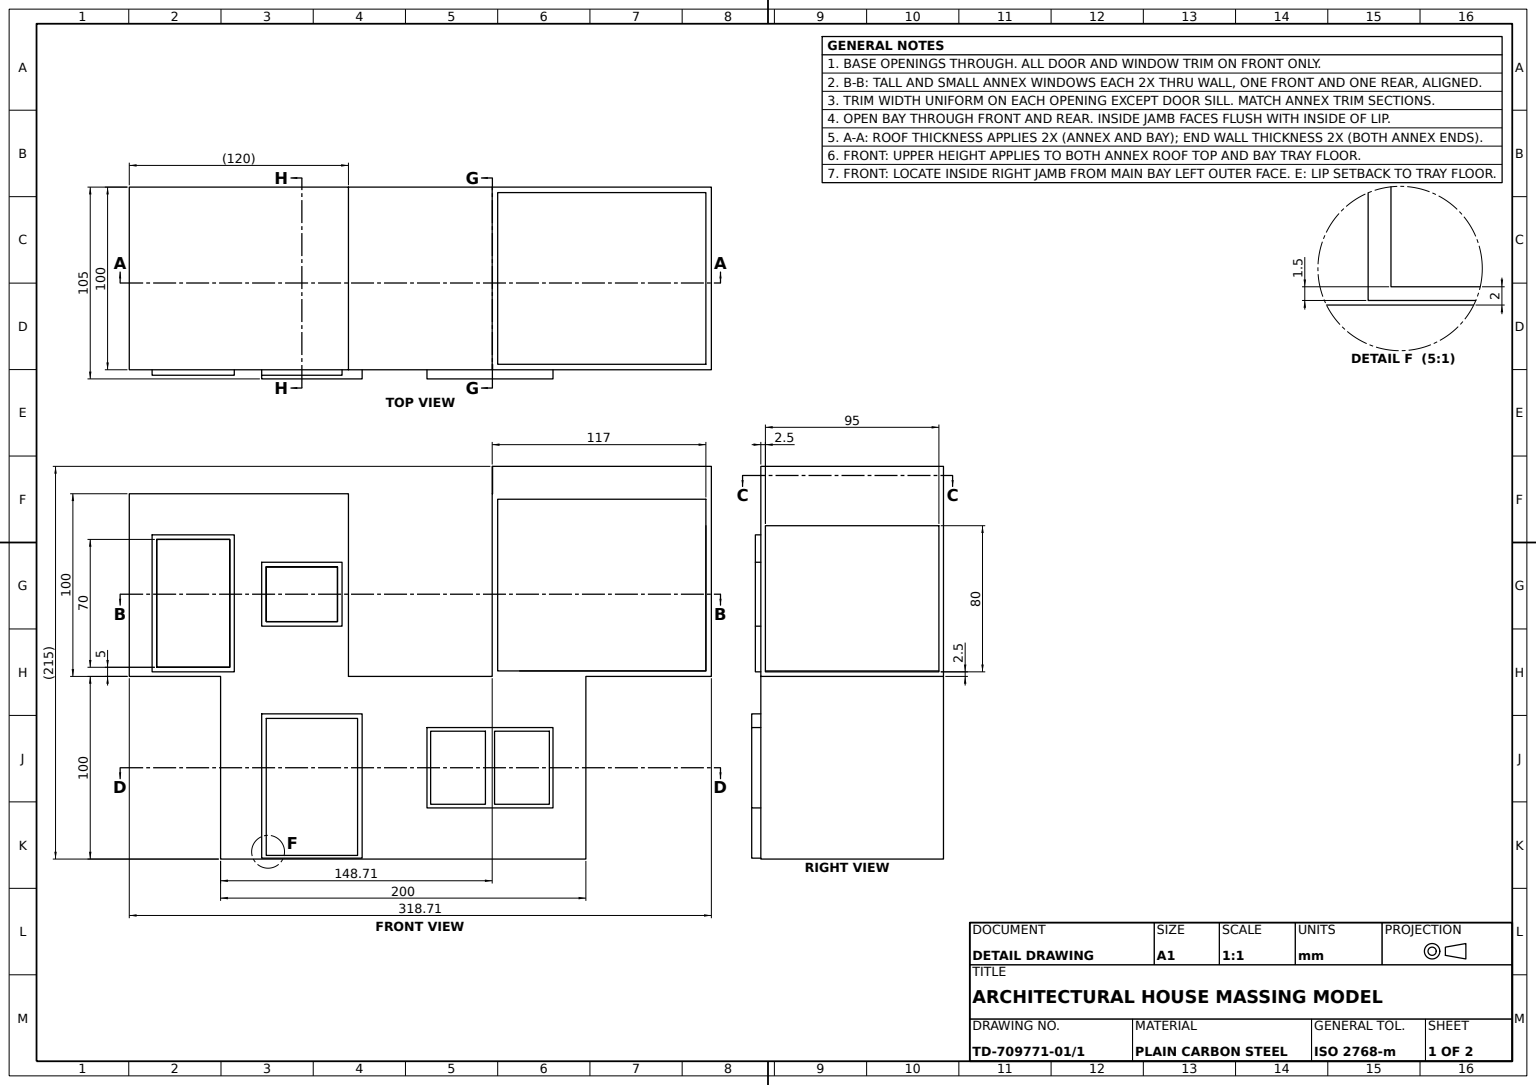
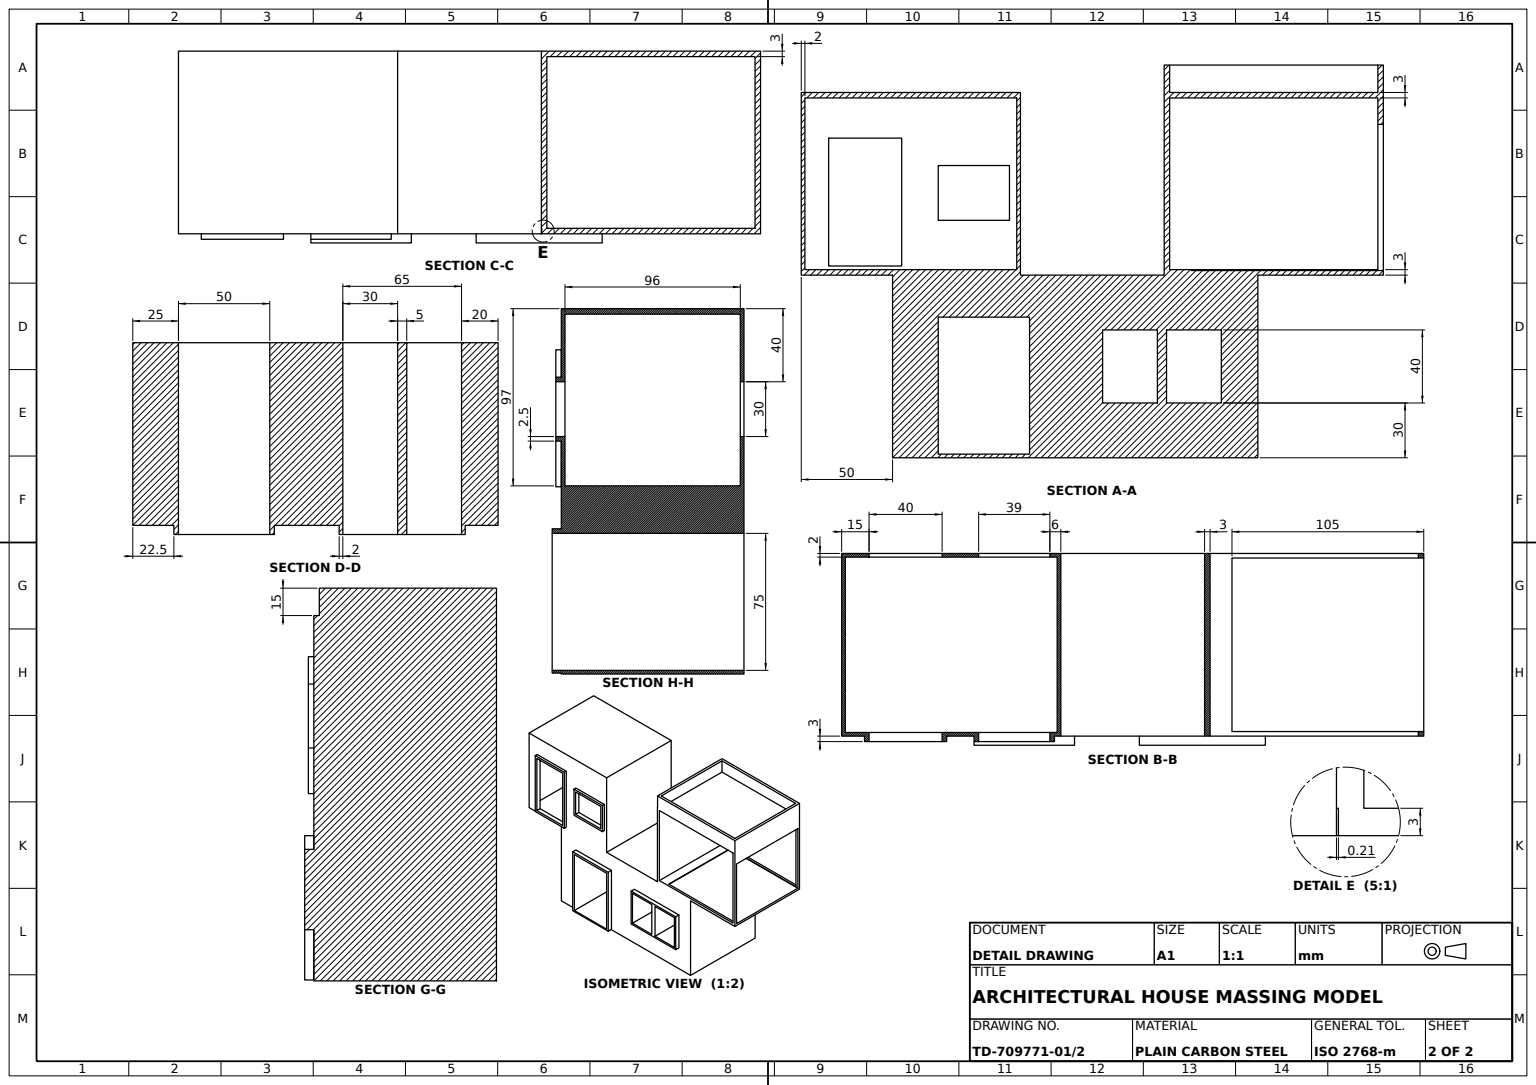
from build123d import *

# Parameters (mm, degrees)
BASE_BLOCK_SKETCH_W           = 200
BASE_BLOCK_SKETCH_H           = 100
BASE_BLOCK_DEPTH              = 100
UPPER_BLOCK_SKETCH_W          = 120
UPPER_BLOCK_SKETCH_H          = 100
UPPER_BLOCK_DEPTH             = 100
SIDE_ANNEX_DEPTH              = 100
FRONT_DOOR_OPENING_SKETCH_W   = 50
FRONT_DOOR_OPENING_SKETCH_H   = 75
FRONT_DOOR_OPENING_DEPTH      = 100
FRONT_WINDOW_OPENING_SKETCH_W = 65
FRONT_WINDOW_OPENING_SKETCH_H = 40
FRONT_WINDOW_OPENING_DEPTH    = 100
FRONT_WINDOW_MULLION_SKETCH_W = 5
FRONT_WINDOW_MULLION_SKETCH_H = 40
FRONT_WINDOW_MULLION_DEPTH    = 100
FRONT_WINDOW_FRAME_SKETCH_W   = 69
FRONT_WINDOW_FRAME_SKETCH_H   = 44
FRONT_WINDOW_FRAME_SKETCH_W_2 = 30
FRONT_WINDOW_FRAME_SKETCH_H_2 = 40
FRONT_WINDOW_FRAME_DEPTH      = 5
FRONT_DOOR_FRAME_SKETCH_W     = 55
FRONT_DOOR_FRAME_SKETCH_H     = 79
FRONT_DOOR_FRAME_SKETCH_W_2   = 50
FRONT_DOOR_FRAME_SKETCH_H_2   = 75
FRONT_DOOR_FRAME_DEPTH        = 5
UPPER_BLOCK_HOLLOW_SKETCH_W   = 114
UPPER_BLOCK_HOLLOW_SKETCH_H   = 94
UPPER_BLOCK_HOLLOW_DEPTH      = 125
UPPER_INTERIOR_CUT_SKETCH_W   = 95
UPPER_INTERIOR_CUT_SKETCH_H   = 80
UPPER_INTERIOR_CUT_DEPTH      = 105
UPPER_FRAME_MEMBER_1_SKETCH_W = 100
UPPER_FRAME_MEMBER_1_SKETCH_H = 15
UPPER_FRAME_MEMBER_1_DEPTH    = 3
UPPER_FRAME_MEMBER_2_SKETCH_W = 116.787548914
UPPER_FRAME_MEMBER_2_SKETCH_H = 15
UPPER_FRAME_MEMBER_2_DEPTH    = 3
UPPER_FRAME_MEMBER_3_SKETCH_W = 97
UPPER_FRAME_MEMBER_3_SKETCH_H = 15
UPPER_FRAME_MEMBER_3_DEPTH    = 3
UPPER_FRAME_MEMBER_4_SKETCH_W = 114
UPPER_FRAME_MEMBER_4_SKETCH_H = 15
UPPER_FRAME_MEMBER_4_DEPTH    = 3
ANNEX_DOOR_OPENING_SKETCH_W   = 40
ANNEX_DOOR_OPENING_SKETCH_H   = 70
ANNEX_DOOR_OPENING_DEPTH      = 153
ANNEX_WINDOW_OPENING_SKETCH_W = 39
ANNEX_WINDOW_OPENING_SKETCH_H = 30
ANNEX_WINDOW_OPENING_DEPTH    = 153
ANNEX_DOOR_FRAME_SKETCH_W     = 45
ANNEX_DOOR_FRAME_SKETCH_H     = 75
ANNEX_DOOR_FRAME_SKETCH_W_2   = 40
ANNEX_DOOR_FRAME_SKETCH_H_2   = 70
ANNEX_DOOR_FRAME_DEPTH        = 3
ANNEX_WINDOW_FRAME_SKETCH_W   = 44
ANNEX_WINDOW_FRAME_SKETCH_H   = 35
ANNEX_WINDOW_FRAME_SKETCH_W_2 = 39
ANNEX_WINDOW_FRAME_SKETCH_H_2 = 30
ANNEX_WINDOW_FRAME_DEPTH      = 3
ANNEX_HOLLOW_SKETCH_W         = 116
ANNEX_HOLLOW_SKETCH_H         = 96
ANNEX_HOLLOW_DEPTH            = 97
ANNEX_RIM_SKETCH_W            = 120
ANNEX_RIM_SKETCH_H            = 100
ANNEX_RIM_DEPTH               = 3


with BuildPart() as part:
    # Base Block Sketch → Base Block (new body)
    with BuildSketch(Plane(origin=(0, 0, 0), x_dir=(1, 0, 0), z_dir=(0, 1, 0))):
        with Locations((100, 50)):
            Rectangle(BASE_BLOCK_SKETCH_W, BASE_BLOCK_SKETCH_H)
    extrude(amount=BASE_BLOCK_DEPTH)

    # Upper Block Sketch → Upper Block (add)
    with BuildSketch(Plane(origin=(0, 100, 0), x_dir=(1, 0, 0), z_dir=(0, 1, 0))):
        with Locations((208.708454776, 50)):
            Rectangle(UPPER_BLOCK_SKETCH_W, UPPER_BLOCK_SKETCH_H)
    extrude(amount=UPPER_BLOCK_DEPTH)

    # Side Annex Sketch → Side Annex (add)
    with BuildSketch(Plane(origin=(0, 100, 0), x_dir=(1, 0, 0), z_dir=(0, 1, 0))):
        Polygon((0, 0), (70, 0), (70, 100), (0, 100), (-50, 100), (-50, 0), align=None)
    extrude(amount=SIDE_ANNEX_DEPTH)

    # Front Door Opening Sketch → Front Door Opening (cut)
    with BuildSketch(Plane.XY):
        with Locations((50, 39.5)):
            Rectangle(FRONT_DOOR_OPENING_SKETCH_W, FRONT_DOOR_OPENING_SKETCH_H)
    extrude(amount=-FRONT_DOOR_OPENING_DEPTH, mode=Mode.SUBTRACT)

    # Front Window Opening Sketch → Front Window Opening (cut)
    with BuildSketch(Plane.XY):
        with Locations((147.5, 50)):
            Rectangle(FRONT_WINDOW_OPENING_SKETCH_W, FRONT_WINDOW_OPENING_SKETCH_H)
    extrude(amount=-FRONT_WINDOW_OPENING_DEPTH, mode=Mode.SUBTRACT)

    # Front Window Mullion Sketch → Front Window Mullion (add)
    with BuildSketch(Plane.XY):
        with Locations((147.5, 50)):
            Rectangle(FRONT_WINDOW_MULLION_SKETCH_W, FRONT_WINDOW_MULLION_SKETCH_H)
    extrude(amount=-FRONT_WINDOW_MULLION_DEPTH)

    # Front Window Frame Sketch → Front Window Frame (add)
    with BuildSketch(Plane.XY):
        with Locations((147.5, 50)):
            Rectangle(FRONT_WINDOW_FRAME_SKETCH_W, FRONT_WINDOW_FRAME_SKETCH_H)
        with Locations((130, 50)):
            Rectangle(FRONT_WINDOW_FRAME_SKETCH_W_2, FRONT_WINDOW_FRAME_SKETCH_H_2, mode=Mode.SUBTRACT)
        with Locations((165, 50)):
            Rectangle(FRONT_WINDOW_FRAME_SKETCH_W_2, FRONT_WINDOW_FRAME_SKETCH_H_2, mode=Mode.SUBTRACT)
    extrude(amount=FRONT_WINDOW_FRAME_DEPTH)

    # Front Door Frame Sketch → Front Door Frame (add)
    with BuildSketch(Plane.XY):
        with Locations((50, 40)):
            Rectangle(FRONT_DOOR_FRAME_SKETCH_W, FRONT_DOOR_FRAME_SKETCH_H)
        with Locations((50, 39.5)):
            Rectangle(FRONT_DOOR_FRAME_SKETCH_W_2, FRONT_DOOR_FRAME_SKETCH_H_2, mode=Mode.SUBTRACT)
    extrude(amount=FRONT_DOOR_FRAME_DEPTH)

    # Upper Block Hollow Sketch → Upper Block Hollow (cut)
    with BuildSketch(Plane.XY):
        with Locations((208.708454776, 150)):
            Rectangle(UPPER_BLOCK_HOLLOW_SKETCH_W, UPPER_BLOCK_HOLLOW_SKETCH_H)
    extrude(amount=-UPPER_BLOCK_HOLLOW_DEPTH, mode=Mode.SUBTRACT)

    # Upper Interior Cut Sketch → Upper Interior Cut (cut)
    with BuildSketch(Plane(origin=(268.708454776, 0, 0), x_dir=(0, 0, -1), z_dir=(1, 0, 0))):
        with Locations((50, 142.5)):
            Rectangle(UPPER_INTERIOR_CUT_SKETCH_W, UPPER_INTERIOR_CUT_SKETCH_H)
    extrude(amount=-UPPER_INTERIOR_CUT_DEPTH, mode=Mode.SUBTRACT)

    # Upper Frame Member 1 Sketch → Upper Frame Member 1 (add)
    with BuildSketch(Plane(origin=(268.708454776, 0, 0), x_dir=(0, 0, -1), z_dir=(1, 0, 0))):
        with Locations((50, 207.5)):
            Rectangle(UPPER_FRAME_MEMBER_1_SKETCH_W, UPPER_FRAME_MEMBER_1_SKETCH_H)
    extrude(amount=-UPPER_FRAME_MEMBER_1_DEPTH)

    # Upper Frame Member 2 Sketch → Upper Frame Member 2 (add)
    with BuildSketch(Plane.XY):
        with Locations((207.314680319, 207.5)):
            Rectangle(UPPER_FRAME_MEMBER_2_SKETCH_W, UPPER_FRAME_MEMBER_2_SKETCH_H)
    extrude(amount=-UPPER_FRAME_MEMBER_2_DEPTH)

    # Upper Frame Member 3 Sketch → Upper Frame Member 3 (add)
    with BuildSketch(Plane.ZY.offset(-148.708454776)):
        with Locations((-51.5, 207.5)):
            Rectangle(UPPER_FRAME_MEMBER_3_SKETCH_W, UPPER_FRAME_MEMBER_3_SKETCH_H)
    extrude(amount=-UPPER_FRAME_MEMBER_3_DEPTH)

    # Upper Frame Member 4 Sketch → Upper Frame Member 4 (add)
    with BuildSketch(Plane(origin=(0, 0, -100), x_dir=(-1, 0, 0), z_dir=(0, 0, -1))):
        with Locations((-208.708454776, 207.5)):
            Rectangle(UPPER_FRAME_MEMBER_4_SKETCH_W, UPPER_FRAME_MEMBER_4_SKETCH_H)
    extrude(amount=-UPPER_FRAME_MEMBER_4_DEPTH)

    # Annex Door Opening Sketch → Annex Door Opening (cut)
    with BuildSketch(Plane.XY):
        with Locations((-15, 140)):
            Rectangle(ANNEX_DOOR_OPENING_SKETCH_W, ANNEX_DOOR_OPENING_SKETCH_H)
    extrude(amount=-ANNEX_DOOR_OPENING_DEPTH, mode=Mode.SUBTRACT)

    # Annex Window Opening Sketch → Annex Window Opening (cut)
    with BuildSketch(Plane.XY):
        with Locations((44.5, 145)):
            Rectangle(ANNEX_WINDOW_OPENING_SKETCH_W, ANNEX_WINDOW_OPENING_SKETCH_H)
    extrude(amount=-ANNEX_WINDOW_OPENING_DEPTH, mode=Mode.SUBTRACT)

    # Annex Door Frame Sketch → Annex Door Frame (add)
    with BuildSketch(Plane.XY):
        with Locations((-15, 140)):
            Rectangle(ANNEX_DOOR_FRAME_SKETCH_W, ANNEX_DOOR_FRAME_SKETCH_H)
        with Locations((-15, 140)):
            Rectangle(ANNEX_DOOR_FRAME_SKETCH_W_2, ANNEX_DOOR_FRAME_SKETCH_H_2, mode=Mode.SUBTRACT)
    extrude(amount=ANNEX_DOOR_FRAME_DEPTH)

    # Annex Window Frame Sketch → Annex Window Frame (add)
    with BuildSketch(Plane.XY):
        with Locations((44.5, 145)):
            Rectangle(ANNEX_WINDOW_FRAME_SKETCH_W, ANNEX_WINDOW_FRAME_SKETCH_H)
        with Locations((44.5, 145)):
            Rectangle(ANNEX_WINDOW_FRAME_SKETCH_W_2, ANNEX_WINDOW_FRAME_SKETCH_H_2, mode=Mode.SUBTRACT)
    extrude(amount=ANNEX_WINDOW_FRAME_DEPTH)

    # Annex Hollow Sketch → Annex Hollow (cut)
    with BuildSketch(Plane(origin=(0, 200, 0), x_dir=(1, 0, 0), z_dir=(0, 1, 0))):
        with Locations((10, 50)):
            Rectangle(ANNEX_HOLLOW_SKETCH_W, ANNEX_HOLLOW_SKETCH_H)
    extrude(amount=-ANNEX_HOLLOW_DEPTH, mode=Mode.SUBTRACT)

    # Annex Rim Sketch → Annex Rim (add)
    with BuildSketch(Plane(origin=(0, 200, 0), x_dir=(1, 0, 0), z_dir=(0, 1, 0))):
        with Locations((10, 50)):
            Rectangle(ANNEX_RIM_SKETCH_W, ANNEX_RIM_SKETCH_H)
    extrude(amount=-ANNEX_RIM_DEPTH)


solid = part.part
